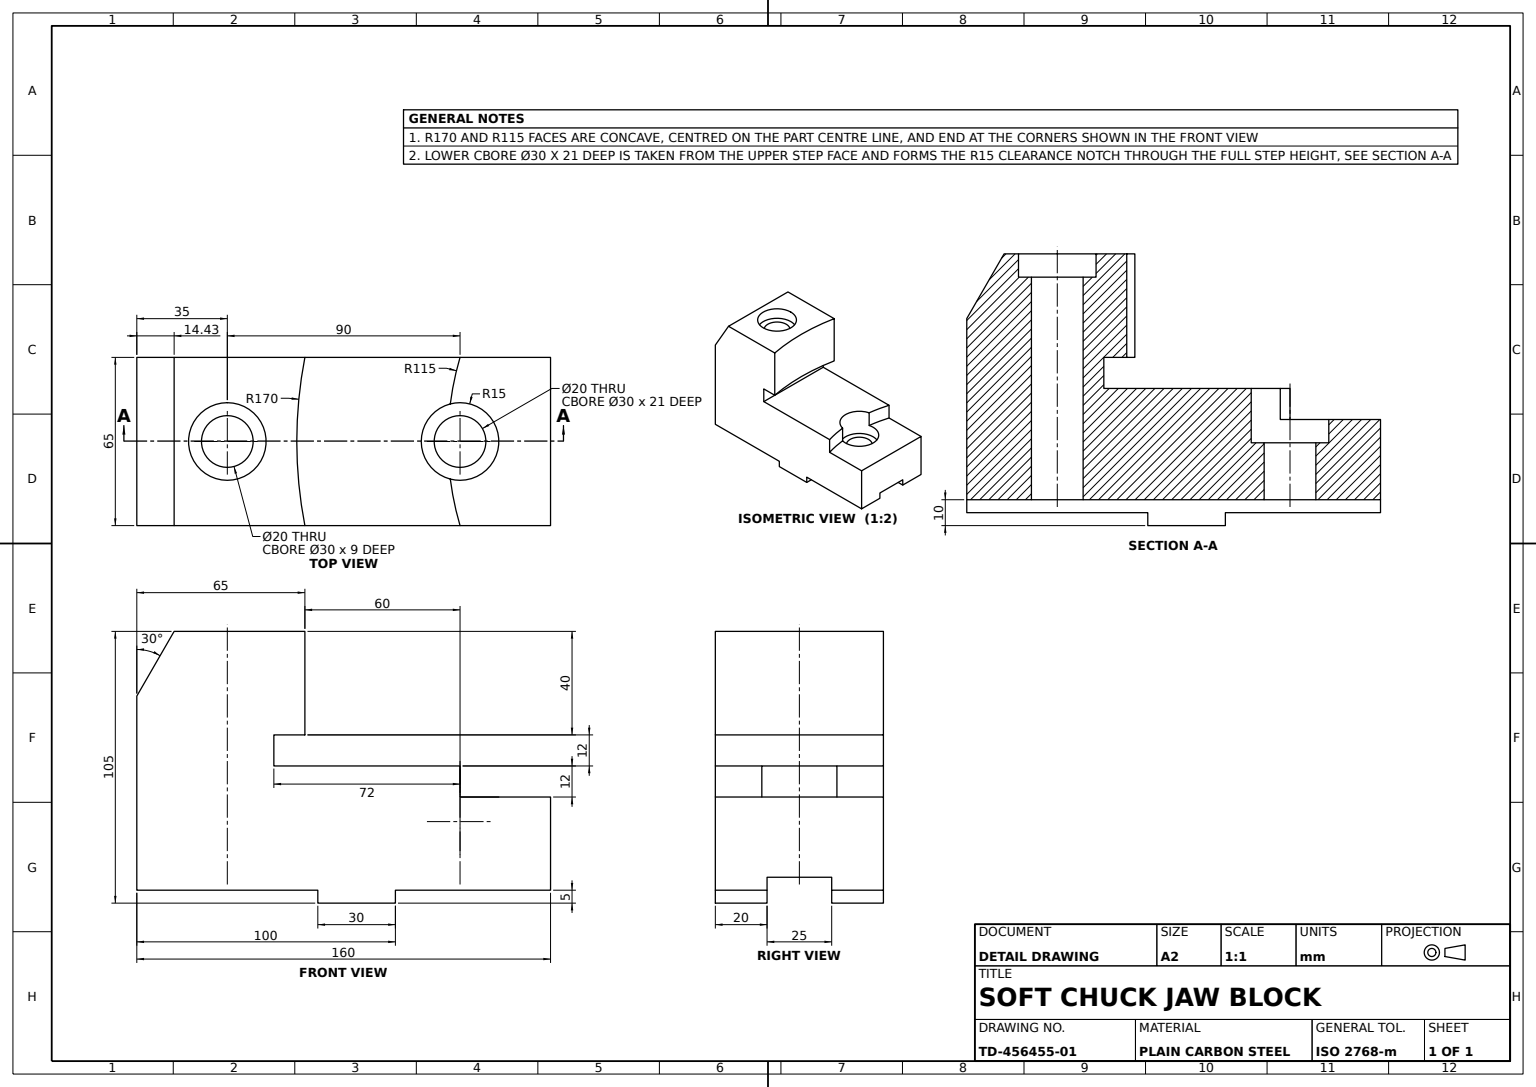
from build123d import *

# Parameters (mm, degrees)
STEPPED_BLOCK_BODY_DEPTH         = 65
RELIEF_CUT_20X20_DEPTH           = 200.562020435
ARC_CUT_115_SKETCH_R             = 115
ARC_CUT_115_DEPTH                = 12
ARC_CUT_170_SKETCH_R             = 170
ARC_CUT_170_DEPTH                = 40
LOWER_C_BORE_HOLE_20_D           = 20
LOWER_C_BORE_HOLE_20_DEPTH       = 99.874921777
LOWER_C_BORE_HOLE_20_CBORE_D     = 30
LOWER_C_BORE_HOLE_20_CBORE_DEPTH = 9
HOLE_CLEARANCE_NOTCH_SKETCH_R    = 15
HOLE_CLEARANCE_NOTCH_DEPTH       = 12


with BuildPart() as part:
    # Stepped Profile Sketch → Stepped Block Body (new body)
    with BuildSketch(Plane.XY):
        Polygon((0, 0), (0, 75), (14.43375673, 100), (65, 100), (65, 60), (53, 60), (53, 48), (65, 48), (125, 48), (125, 36), (160, 36), (160, 0), (100, 0), (100, -5), (70, -5), (70, 0), align=None)
    extrude(amount=STEPPED_BLOCK_BODY_DEPTH)

    # Relief Cut Sketch → Relief Cut 20x20 (cut, through all)
    with BuildSketch(Plane(origin=(160, 0, 0), x_dir=(0, 0, -1), z_dir=(1, 0, 0))):
        Polygon((-45, 0), (-45, 5), (-20, 5), (-20, 0), (-20, -9.038328121), (-45, -9.038328121), align=None)
    extrude(amount=-RELIEF_CUT_20X20_DEPTH, mode=Mode.SUBTRACT)

    # Arc Cut 115 Sketch → Arc Cut 115 (cut)
    with BuildSketch(Plane(origin=(0, 48, 0), x_dir=(1, 0, 0), z_dir=(0, 1, 0))):
        with Locations((235.312057365, -32.5)):
            Circle(ARC_CUT_115_SKETCH_R)
    extrude(amount=-ARC_CUT_115_DEPTH, mode=Mode.SUBTRACT)

    # Arc Cut 170 Sketch → Arc Cut 170 (cut)
    with BuildSketch(Plane(origin=(0, 100, 0), x_dir=(1, 0, 0), z_dir=(0, 1, 0))):
        with Locations((231.86446596, -32.5)):
            Circle(ARC_CUT_170_SKETCH_R)
    extrude(amount=-ARC_CUT_170_DEPTH, mode=Mode.SUBTRACT)

    # Sketch11 → Upper C-Bore Hole Ø20 (revolve, cut)
    with BuildSketch(Plane(origin=(125, 36, 32.5), x_dir=(0, 0, 1), z_dir=(1, 0, 0))):
        Polygon((0, 0), (0, 99.874921777), (10, 99.874921777), (10, 9), (15, 9), (15, 0), align=None)
    revolve(axis=Axis((125, -74, 32.5), (0, 1, 0)), mode=Mode.SUBTRACT)

    # Lower C-Bore Hole Ø20
    with Locations(Plane(origin=(35, 100, 32.5), x_dir=(1, 0, 0), z_dir=(0, 1, 0))):
        with Locations((0, 0)):
            CounterBoreHole(LOWER_C_BORE_HOLE_20_D / 2, LOWER_C_BORE_HOLE_20_CBORE_D / 2, LOWER_C_BORE_HOLE_20_CBORE_DEPTH, depth=LOWER_C_BORE_HOLE_20_DEPTH)

    # Hole Clearance Notch Sketch → Hole Clearance Notch (cut)
    with BuildSketch(Plane(origin=(0, 48, 0), x_dir=(1, 0, 0), z_dir=(0, 1, 0))):
        with Locations(Location((125, -32.5, 0), (0, 0, 270))):
            Circle(HOLE_CLEARANCE_NOTCH_SKETCH_R)
    extrude(amount=-HOLE_CLEARANCE_NOTCH_DEPTH, mode=Mode.SUBTRACT)


solid = part.part
